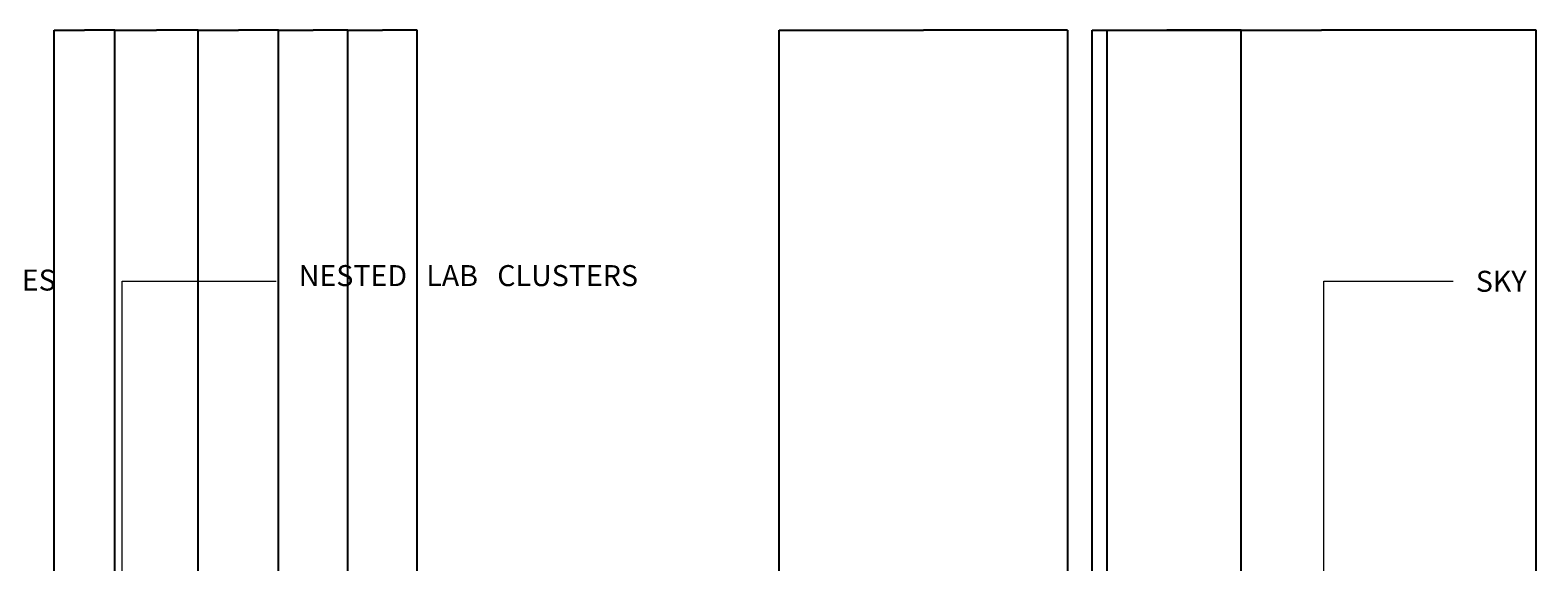
# Model space of a CAD drawing. Units: inches. Extents: x -32109 to 33221, y -19197 to 7608.
# Tile 7 of 25: x -12087 to -741, y -11338 to -7335. Entities that reach past the tile are written whole.
import ezdxf

# ---------------------------------------------------------------- set-up
doc = ezdxf.new("R2010")
doc.units = ezdxf.units.IN
doc.header["$MEASUREMENT"] = 0
for name, color, linetype, lineweight in [('A-ANNO-DIMS', 2, 'Continuous', 18), ('A-ANNO-NOTE', 2, 'Continuous', 18), ('A-ANNO-TEXT', 7, 'Continuous', 25)]:
    doc.layers.add(name, color=color, linetype=linetype, lineweight=lineweight)
doc.styles.get("Standard").update_dxf_attribs({"font": 'arial.ttf'})
doc.dimstyles.get("Standard").update_dxf_attribs({"dimtxt": 0.18, "dimasz": 0.18, "dimexe": 0.18, "dimexo": 0.0625, "dimgap": 0.09, "dimtad": 0, "dimtih": 1, "dimtoh": 1, "dimdec": 4, "dimzin": 0, "dimdsep": 46, "dimtxsty": 'Standard', "dimcen": 0.09, "dimadec": 0, "dimazin": 0, "dimtfac": 1, "dimtdec": 4, "dimtofl": 0, "dimtmove": 0, "dimatfit": 3, "dimfxl": 1, "dimtolj": 1, "dimtzin": 0, "dimarcsym": 0})

# ---------------------------------------------------------------- blocks, each defined once
blk = doc.blocks.new('*D14')
at = {"layer": 'A-ANNO-DIMS', "color": 0, "lineweight": -2, "transparency": 16777216}
for p, q in [((-18893.90707200001, -10978.730223), (-32108.36667400003, -10978.73022300001)), ((-32108.18667400003, -10978.91022300001), (-32108.18667400003, -13611.23962386222)), ((-32108.18667400003, -16243.93283100001), (-32108.18667400003, -13611.6034301378)), ((5067.088884000002, -16244.11283100001), (-32108.36667400003, -16244.11283100001))]:
    blk.add_line(p, q, dxfattribs=at)
at = {"layer": 'A-ANNO-DIMS', "color": 0, "transparency": 16777216}
for points in [[(-32108.21667400003, -10978.91022300001), (-32108.15667400003, -10978.91022300001), (-32108.18667400003, -10978.73022300001)], [(-32108.21667400003, -16243.93283100001), (-32108.15667400003, -16243.93283100001), (-32108.18667400003, -16244.11283100001)]]:
    blk.add_solid(points, dxfattribs=at)
at = {"layer": 'Defpoints', "color": 0, "transparency": 16777216}
for p in [(-18893.84457200001, -10978.730223), (-32108.18667400003, -16244.11283100001), (5067.151384000002, -16244.11283100001)]:
    blk.add_point(p, dxfattribs=at)
at = {"layer": 'A-ANNO-DIMS', "color": 0, "transparency": 16777216, "insert": (-32108.18667400002, -13611.421527), "char_height": 0.18, "attachment_point": 5}
blk.add_mtext('\\A1;5265', dxfattribs=at)
blk = doc.blocks.new('*D22')
at = {"layer": 'A-ANNO-DIMS', "color": 0, "lineweight": -2, "transparency": 16777216}
for p, q in [((-4093.675456999999, -14968.01648), (-4093.675456999999, -7334.980009999999)), ((-4093.495456999999, -7335.16001), (-3534.410175540246, -7335.16001)), ((-2974.415317, -7335.16001), (-3533.500598459754, -7335.16001)), ((-2974.235317, -14968.01648), (-2974.235317, -7334.980009999999))]:
    blk.add_line(p, q, dxfattribs=at)
at = {"layer": 'A-ANNO-DIMS', "color": 0, "transparency": 16777216}
for points in [[(-4093.495456999999, -7335.13001), (-4093.495456999999, -7335.190009999999), (-4093.675456999999, -7335.16001)], [(-2974.415317, -7335.13001), (-2974.415317, -7335.190009999999), (-2974.235317, -7335.16001)]]:
    blk.add_solid(points, dxfattribs=at)
at = {"layer": 'Defpoints', "color": 0, "transparency": 16777216}
for p in [(-2974.235317, -7335.16001), (-4093.675456999999, -14968.07898), (-2974.235317, -14968.07898)]:
    blk.add_point(p, dxfattribs=at)
at = {"layer": 'A-ANNO-DIMS', "color": 0, "transparency": 16777216, "insert": (-3533.955387, -7335.16001), "char_height": 0.18, "attachment_point": 5}
blk.add_mtext('\\A1;1119.4', dxfattribs=at)
blk = doc.blocks.new('*D94')
at = {"layer": 'A-ANNO-DIMS', "color": 0, "lineweight": -2, "transparency": 16777216}
for p, q in [((-11907.663717, -13728.965541), (-11907.663717, -7334.980009999999)), ((-11907.483717, -7335.16001), (-11679.46514968417, -7335.16001)), ((-11450.653772, -7335.16001), (-11678.67233931582, -7335.16001)), ((-11450.473772, -13728.965541), (-11450.473772, -7334.980009999999))]:
    blk.add_line(p, q, dxfattribs=at)
at = {"layer": 'A-ANNO-DIMS', "color": 0, "transparency": 16777216}
for points in [[(-11907.483717, -7335.13001), (-11907.483717, -7335.190009999999), (-11907.663717, -7335.16001)], [(-11450.653772, -7335.13001), (-11450.653772, -7335.190009999999), (-11450.473772, -7335.16001)]]:
    blk.add_solid(points, dxfattribs=at)
at = {"layer": 'Defpoints', "color": 0, "transparency": 16777216}
for p in [(-11450.473772, -7335.16001), (-11907.663717, -13729.028041), (-11450.473772, -13729.028041)]:
    blk.add_point(p, dxfattribs=at)
at = {"layer": 'A-ANNO-DIMS', "color": 0, "transparency": 16777216, "insert": (-11679.0687445, -7335.16001), "char_height": 0.18, "attachment_point": 5}
blk.add_mtext('\\A1;457.2', dxfattribs=at)
blk = doc.blocks.new('*D95')
at = {"layer": 'A-ANNO-DIMS', "color": 0, "lineweight": -2, "transparency": 16777216}
for p, q in [((-11450.473772, -13728.965541), (-11450.473772, -7334.980009999999)), ((-11450.293772, -7335.16001), (-11137.21442408867, -7335.16001)), ((-10823.346686, -7335.16001), (-11136.42603391132, -7335.16001)), ((-10823.166686, -13728.965541), (-10823.166686, -7334.980009999999))]:
    blk.add_line(p, q, dxfattribs=at)
at = {"layer": 'A-ANNO-DIMS', "color": 0, "transparency": 16777216}
for points in [[(-11450.293772, -7335.13001), (-11450.293772, -7335.190009999999), (-11450.473772, -7335.16001)], [(-10823.346686, -7335.13001), (-10823.346686, -7335.190009999999), (-10823.166686, -7335.16001)]]:
    blk.add_solid(points, dxfattribs=at)
at = {"layer": 'Defpoints', "color": 0, "transparency": 16777216}
for p in [(-10823.166686, -7335.16001), (-11450.473772, -13729.028041), (-10823.166686, -13729.028041)]:
    blk.add_point(p, dxfattribs=at)
at = {"layer": 'A-ANNO-DIMS', "color": 0, "transparency": 16777216, "insert": (-11136.820229, -7335.16001), "char_height": 0.18, "attachment_point": 5}
blk.add_mtext('\\A1;627.3', dxfattribs=at)
blk = doc.blocks.new('*D96')
at = {"layer": 'A-ANNO-DIMS', "color": 0, "lineweight": -2, "transparency": 16777216}
for p, q in [((-10823.166686, -13728.965541), (-10823.166686, -7334.980009999999)), ((-10822.986686, -7335.16001), (-10520.43466844406, -7335.16001)), ((-10217.304097, -7335.16001), (-10519.85611455593, -7335.16001)), ((-10217.124097, -13728.965541), (-10217.124097, -7334.980009999999))]:
    blk.add_line(p, q, dxfattribs=at)
at = {"layer": 'A-ANNO-DIMS', "color": 0, "transparency": 16777216}
for points in [[(-10822.986686, -7335.13001), (-10822.986686, -7335.190009999999), (-10823.166686, -7335.16001)], [(-10217.304097, -7335.13001), (-10217.304097, -7335.190009999999), (-10217.124097, -7335.16001)]]:
    blk.add_solid(points, dxfattribs=at)
at = {"layer": 'Defpoints', "color": 0, "transparency": 16777216}
for p in [(-10217.124097, -7335.16001), (-10823.166686, -13729.028041), (-10217.124097, -13729.028041)]:
    blk.add_point(p, dxfattribs=at)
at = {"layer": 'A-ANNO-DIMS', "color": 0, "transparency": 16777216, "insert": (-10520.1453915, -7335.16001), "char_height": 0.18, "attachment_point": 5}
blk.add_mtext('\\A1;606', dxfattribs=at)
blk = doc.blocks.new('*D97')
at = {"layer": 'A-ANNO-DIMS', "color": 0, "lineweight": -2, "transparency": 16777216}
for p, q in [((-10217.124097, -13728.965541), (-10217.124097, -7334.980009999999)), ((-10216.944097, -7335.16001), (-9956.903619396999, -7335.16001)), ((-9696.320195, -7335.16001), (-9956.360672603001, -7335.16001)), ((-9696.140194999998, -13728.965541), (-9696.140194999998, -7334.980009999999))]:
    blk.add_line(p, q, dxfattribs=at)
at = {"layer": 'A-ANNO-DIMS', "color": 0, "transparency": 16777216}
for points in [[(-10216.944097, -7335.13001), (-10216.944097, -7335.190009999999), (-10217.124097, -7335.16001)], [(-9696.320195, -7335.13001), (-9696.320195, -7335.190009999999), (-9696.140194999998, -7335.16001)]]:
    blk.add_solid(points, dxfattribs=at)
at = {"layer": 'Defpoints', "color": 0, "transparency": 16777216}
for p in [(-9696.140194999998, -7335.16001), (-10217.124097, -13729.028041), (-9696.140194999998, -13729.028041)]:
    blk.add_point(p, dxfattribs=at)
at = {"layer": 'A-ANNO-DIMS', "color": 0, "transparency": 16777216, "insert": (-9956.632146, -7335.16001), "char_height": 0.18, "attachment_point": 5}
blk.add_mtext('\\A1;521', dxfattribs=at)
blk = doc.blocks.new('*D98')
at = {"layer": 'A-ANNO-DIMS', "color": 0, "lineweight": -2, "transparency": 16777216}
for p, q in [((-9696.140194999998, -13728.965541), (-9696.140194999998, -7334.980009999999)), ((-9695.960195, -7335.16001), (-9435.919834396997, -7335.16001)), ((-9175.336527, -7335.16001), (-9435.376887603, -7335.16001)), ((-9175.156527, -13728.965541), (-9175.156527, -7334.980009999999))]:
    blk.add_line(p, q, dxfattribs=at)
at = {"layer": 'A-ANNO-DIMS', "color": 0, "transparency": 16777216}
for points in [[(-9695.960195, -7335.13001), (-9695.960195, -7335.190009999999), (-9696.140194999998, -7335.16001)], [(-9175.336527, -7335.13001), (-9175.336527, -7335.190009999999), (-9175.156527, -7335.16001)]]:
    blk.add_solid(points, dxfattribs=at)
at = {"layer": 'Defpoints', "color": 0, "transparency": 16777216}
for p in [(-9175.156527, -7335.16001), (-9696.140194999998, -13729.028041), (-9175.156527, -13729.028041)]:
    blk.add_point(p, dxfattribs=at)
at = {"layer": 'A-ANNO-DIMS', "color": 0, "transparency": 16777216, "insert": (-9435.648361, -7335.16001), "char_height": 0.18, "attachment_point": 5}
blk.add_mtext('\\A1;521', dxfattribs=at)
blk = doc.blocks.new('*D108')
at = {"layer": 'A-ANNO-DIMS', "color": 0, "lineweight": -2, "transparency": 16777216}
for p, q in [((-6449.955339, -11850.731733), (-6449.955339, -7334.980009999999)), ((-6449.775339, -7335.16001), (-5364.796697151433, -7335.16001)), ((-4279.132189, -7335.16001), (-5364.110830848567, -7335.16001)), ((-4278.952188999999, -11850.731733), (-4278.952188999999, -7334.980009999999))]:
    blk.add_line(p, q, dxfattribs=at)
at = {"layer": 'A-ANNO-DIMS', "color": 0, "transparency": 16777216}
for points in [[(-6449.775339, -7335.13001), (-6449.775339, -7335.190009999999), (-6449.955339, -7335.16001)], [(-4279.132189, -7335.13001), (-4279.132189, -7335.190009999999), (-4278.952188999999, -7335.16001)]]:
    blk.add_solid(points, dxfattribs=at)
at = {"layer": 'Defpoints', "color": 0, "transparency": 16777216}
for p in [(-4278.952188999999, -7335.16001), (-6449.955339, -11850.794233), (-4278.952188999999, -11850.794233)]:
    blk.add_point(p, dxfattribs=at)
at = {"layer": 'A-ANNO-DIMS', "color": 0, "transparency": 16777216, "insert": (-5364.453764, -7335.16001), "char_height": 0.18, "attachment_point": 5}
blk.add_mtext('\\A1;2171', dxfattribs=at)
blk = doc.blocks.new('*D109')
at = {"layer": 'A-ANNO-DIMS', "color": 0, "lineweight": -2, "transparency": 16777216}
for p, q in [((-3982.394421, -12255.869051), (-3982.394421, -7334.980009999999)), ((-3982.214421, -7335.16001), (-2368.67456495225, -7335.16001)), ((-754.4169189999996, -7335.16001), (-2367.956775047749, -7335.16001)), ((-754.236919, -12255.869051), (-754.2369189999996, -7334.980009999999))]:
    blk.add_line(p, q, dxfattribs=at)
at = {"layer": 'A-ANNO-DIMS', "color": 0, "transparency": 16777216}
for points in [[(-3982.214421, -7335.13001), (-3982.214421, -7335.190009999999), (-3982.394421, -7335.16001)], [(-754.4169189999996, -7335.13001), (-754.4169189999996, -7335.190009999999), (-754.2369189999996, -7335.16001)]]:
    blk.add_solid(points, dxfattribs=at)
at = {"layer": 'Defpoints', "color": 0, "transparency": 16777216}
for p in [(-754.2369189999996, -7335.16001), (-3982.394421, -12255.931551), (-754.236919, -12255.931551)]:
    blk.add_point(p, dxfattribs=at)
at = {"layer": 'A-ANNO-DIMS', "color": 0, "transparency": 16777216, "insert": (-2368.315669999999, -7335.16001), "char_height": 0.18, "attachment_point": 5}
blk.add_mtext('\\A1;3228', dxfattribs=at)

msp = doc.modelspace()

# ---------------------------------------------------------------- linework, layer by layer
at = {"layer": 'A-ANNO-NOTE'}
for p, q in [((-11395.93241528085, -11625.26732475804), (-11395.93241528085, -9225.160009906325)), ((-11395.93241528085, -9225.160009906325), (-10235.31946681617, -9225.160009906325)), ((-2350.305342373555, -11867.63396145224), (-2350.305342373685, -9225.160009906325)), ((-2350.305342373685, -9225.160009906325), (-1378.630045300353, -9225.160009906325))]:
    msp.add_line(p, q, dxfattribs=at)

# ---------------------------------------------------------------- texts
at = {"layer": 'A-ANNO-TEXT'}
for s, p in [('FACADE   SUNSHADES', (-14092.13692296132, -9295.288439036824)), ('NESTED   LAB   CLUSTERS', (-10065.91868563277, -9261.736315729882)), ('SKY   BRIDGE   CONNECTIONS', (-1207.497713132039, -9304.611995487214))]:
    msp.add_text(s, height=157.8985042017455, dxfattribs=at).set_placement(p)

# ---------------------------------------------------------------- dimensions: what is measured, and where the dimension line sits
at = {"layer": 'A-ANNO-DIMS'}
for base, p1, p2, override, picture, middle in [((-11450.473772, -7335.16001), (-11907.663717, -13729.028041), (-11450.473772, -13729.028041), {"dimdec": 1, "dimlfac": 1, "dimrnd": 0, "dimzin": 0, "dimdsep": 46, "dimlunit": 2}, '*D94', (-11679.0687445, -7335.16001)), ((-10823.166686, -7335.16001), (-11450.473772, -13729.028041), (-10823.166686, -13729.028041), {"dimdec": 1, "dimlfac": 1, "dimrnd": 0, "dimzin": 0, "dimdsep": 46, "dimlunit": 2}, '*D95', (-11136.820229, -7335.16001)), ((-10217.124097, -7335.16001), (-10823.166686, -13729.028041), (-10217.124097, -13729.028041), {"dimdec": 0, "dimlfac": 1, "dimrnd": 0, "dimzin": 0, "dimdsep": 46, "dimlunit": 2}, '*D96', (-10520.1453915, -7335.16001)), ((-9696.140194999998, -7335.16001), (-10217.124097, -13729.028041), (-9696.140194999998, -13729.028041), {"dimdec": 0, "dimlfac": 1, "dimrnd": 0, "dimzin": 0, "dimdsep": 46, "dimlunit": 2}, '*D97', (-9956.632146, -7335.16001)), ((-9175.156527, -7335.16001), (-9696.140194999998, -13729.028041), (-9175.156527, -13729.028041), {"dimdec": 0, "dimlfac": 1, "dimrnd": 0, "dimzin": 0, "dimdsep": 46, "dimlunit": 2}, '*D98', (-9435.648361, -7335.16001)), ((-4278.952188999999, -7335.16001), (-6449.955339, -11850.794233), (-4278.952188999999, -11850.794233), {"dimdec": 0, "dimlfac": 1, "dimrnd": 0, "dimzin": 0, "dimdsep": 46, "dimlunit": 2}, '*D108', (-5364.453764, -7335.16001)), ((-2974.235317, -7335.16001), (-4093.675456999999, -14968.07898), (-2974.235317, -14968.07898), {"dimdec": 1, "dimlfac": 1, "dimrnd": 0, "dimzin": 0, "dimdsep": 46, "dimlunit": 2}, '*D22', (-3533.955387, -7335.16001)), ((-754.2369189999996, -7335.16001), (-3982.394421, -12255.931551), (-754.236919, -12255.931551), {"dimdec": 0, "dimlfac": 1, "dimrnd": 0, "dimzin": 0, "dimdsep": 46, "dimlunit": 2}, '*D109', (-2368.315669999999, -7335.16001))]:
    dim = msp.add_linear_dim(base=base, p1=p1, p2=p2, dimstyle='Standard', override=override, dxfattribs=at)
    dim.commit()
    dim.dimension.update_dxf_attribs({"geometry": picture, "text_midpoint": middle})
dim = msp.add_linear_dim(base=(-32108.18667400003, -16244.11283100001), p1=(-18893.844572, -10978.730223), p2=(5067.151383999999, -16244.112831), angle=90, dimstyle='Standard', override={"dimdec": 0, "dimlfac": 1, "dimrnd": 0, "dimzin": 0, "dimdsep": 46, "dimlunit": 2}, dxfattribs=at)
dim.commit()
dim.dimension.update_dxf_attribs({"geometry": '*D14', "text_midpoint": (-32108.18667400002, -13611.421527)})

doc.saveas('drawing.dxf')
